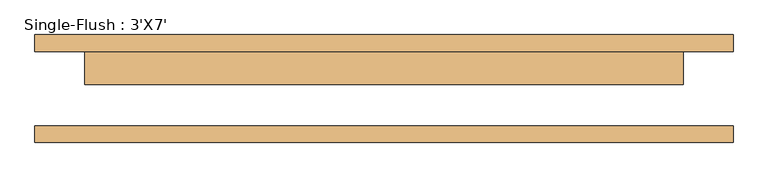
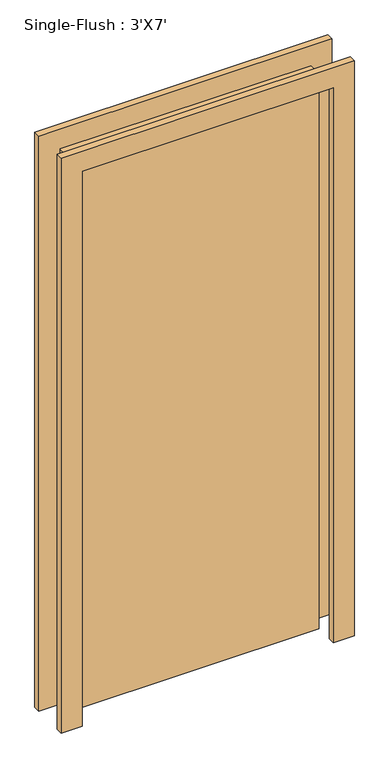
"""IFC4 building model written with IfcOpenShell, lengths in millimetres: door geometry, Single-Flush : 3'X7'."""

from ifc_helpers import new_model, si_unit, frame, origin, origin_with_axes, place, context, project, spatial, polyline, outline, extrude, source, transform, mapped, element, save


def single_flush_3_x7_e5f9f3c4(model_context):
    return source(origin(), model_context, "Body", "SweptSolid", [
        extrude(outline(polyline([(2209.8, -533.4), (0.0, -533.4), (0.0, -457.2), (2133.6, -457.2), (2133.6, 457.2), (0.0, 457.2), (0.0, 533.4), (2209.8, 533.4), (2209.8, -533.4)])), frame((0.0, 57.15, 0.0), z_axis=(0.0, 1.0, 0.0), x_axis=(0.0, 0.0, 1.0)), (0.0, 0.0, 1.0), 25.4),
        extrude(outline(polyline([(2209.8, 533.4), (2209.8, -533.4), (0.0, -533.4), (0.0, -457.2), (2133.6, -457.2), (2133.6, 457.2), (0.0, 457.2), (0.0, 533.4), (2209.8, 533.4)])), frame((0.0, -82.55, 0.0), z_axis=(0.0, 1.0, 0.0), x_axis=(0.0, 0.0, 1.0)), (0.0, 0.0, 1.0), 25.4),
        extrude(outline(polyline([(457.2, 6.35), (-457.2, 6.35), (-457.2, 57.15), (457.2, 57.15), (457.2, 6.35)])), origin_with_axes(), (0.0, 0.0, 1.0), 2133.6),
    ])


if __name__ == "__main__":
    model = new_model("IFC4")
    model_context = context("Model", 3, world=origin())
    ifc_project = project(units=[si_unit("LENGTHUNIT", "METRE", prefix="MILLI")], contexts=[model_context])
    site = spatial("IfcSite", under=ifc_project)
    building = spatial("IfcBuilding", under=site)
    placement = place(None, origin())
    single_flush_3_x7_shape = single_flush_3_x7_e5f9f3c4(model_context)
    element("IfcDoor", 1, ObjectType="Single-Flush : 3'X7'", at=placement, inside=building, context=model_context, shape_type="MappedRepresentation", body=[
        mapped(single_flush_3_x7_shape, transform((0.0, 0.0, 0.0), x_axis=(1.0, 0.0, 0.0), y_axis=(0.0, 1.0, 0.0), z_axis=(0.0, 0.0, 1.0))),
    ])
    save(model, "model.ifc")

# Revit data of these elements
# Type "Single-Flush : 3'X7'"
#   Type Mark = "8"
#   Construction Type Id = "MDOOR"
#   Assembly Code = "C1020"
#   Analytic Construction = "Metal"
#   Thickness = 0' - 2"
#   Heat Transfer Coefficient (U) = 0.651978 BTU/(h·ft²·°F)
#   Height = 7' - 0"
#   Trim Projection Ext = 0' - 1"
#   Trim Projection Int = 0' - 1"
#   Trim Width = 0' - 3"
#   Width = 3' - 0"
#   Define Thermal Properties by = 1
#   Door Material = Door - Panel
#   Frame Material = Door - Frame
#   Visual Light Transmittance = 0
#   Solar Heat Gain Coefficient = 0
#   Function = (empty or 0)
#   Wall Closure = (empty or 0)
# Element 1 (IfcDoor, "Single-Flush : 3'X7'")
#   Materials on its faces: "Door - Frame", "Door - Panel"
# Materials
#   "Door - Panel": class "Wood", colour RGB 210 159 95, transparency 0, Cost = 0
#   "Door - Frame": colour RGB 118 70 51, transparency 0, Cost = 0
